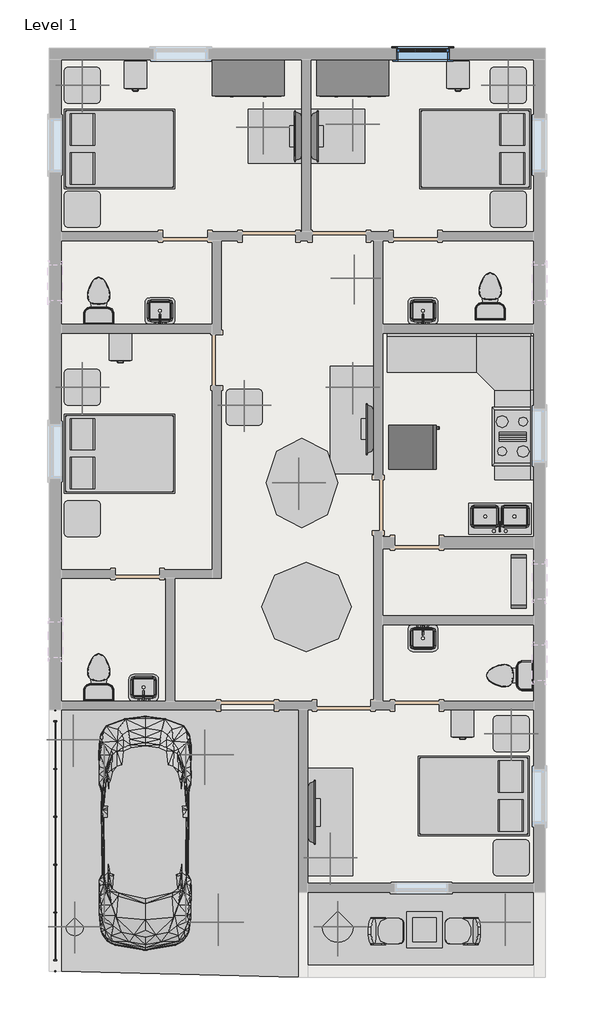
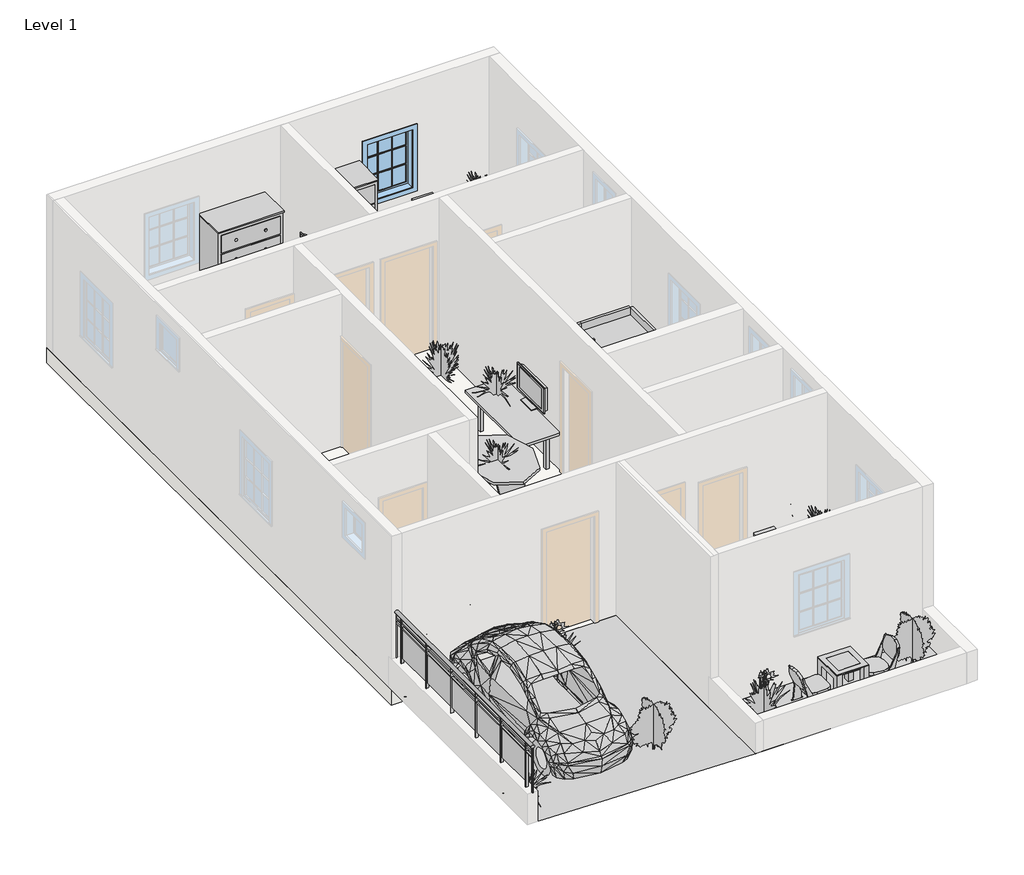
# One storey, part 2 of 2: 34 furniture elements, 17 geographic elements, 13 flow terminals, 5 proxies, 1 railing, 1 slab, 1 window.
# Revit data of these elements (continued)
# Materials (continued)
#   "Laminate, Linen, Matte": class "Plastic", colour RGB 249 239 230, transparency 0, Description = "Plastic Laminate - Linen, Matte", Cost = 0
#   "Birch": class "Wood", colour RGB 224 178 126, transparency 0, Description = "Betula Alleghaniensis", Cost = 0
#   "Linen, White": class "Textile", colour RGB 247 247 239, transparency 0, Description = "Linen, white", Cost = 0
#   "Laminate - Ivory, Glossy": colour RGB 247 247 239, transparency 0
#   "Laminate, Ivory, Matte": class "Plastic", colour RGB 247 247 239, transparency 0, Description = "Plastic Laminate - Ivory, Matte", Cost = 0
#   "Cherry": class "Wood", colour RGB 226 177 128, transparency 0, Description = "Prunus Serotina", Cost = 0
#   "Linen, Beige": class "Textile", colour RGB 249 239 230, transparency 0, Description = "Linen, beige", Cost = 0
#   "Steel, Paint Finish, Dark Gray, Matte": class "Metal", colour RGB 0 0 0, transparency 0, Description = "Steel, paint finish, dark gray, matte", Cost = 0
#   "Pine": class "Wood", colour RGB 223 192 134, transparency 0, Description = "Pinus Echinata", Cost = 0
#   "Textile - Light Gray": class "Fabric", colour RGB 204 204 204, transparency 0
#   "Glass": class "Glass", colour RGB 0 128 192, transparency 0.75, Description = "Soda Lime Glass", Cost = 0
#   "Sash": class "Wood", colour RGB 224 178 126, transparency 0
#   "Trim": class "Wood", colour RGB 224 178 126, transparency 0
#   "TV - Black": colour RGB 49 49 49, transparency 0
#   "TV - Glass": colour RGB 157 157 157, transparency 0.9
#   "TV - Screen": colour RGB 0 0 0, transparency 0
#   "Glass - Clear, Grey": class "Glass", colour RGB 252 255 255, transparency 0.64
#   "Default Floor": colour RGB 128 128 128, transparency 0
